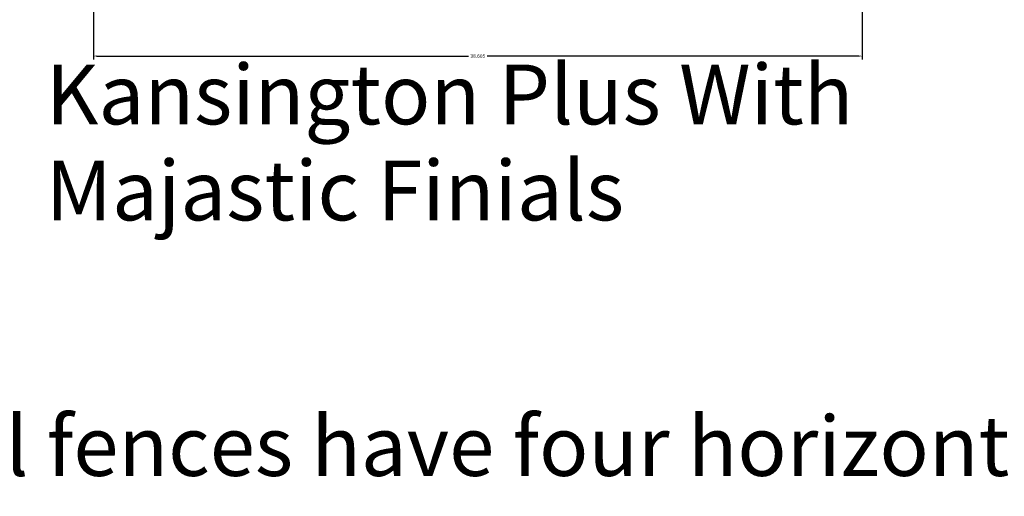
# Model space of a CAD drawing. Units: inches. Extents: x 756 to 915, y 488 to 695.
# Tile 4 of 25: x 813 to 863, y 488 to 512. Entities that reach past the tile are written whole.
import ezdxf

# ---------------------------------------------------------------- set-up
doc = ezdxf.new("R2010")
doc.units = ezdxf.units.IN
doc.header["$MEASUREMENT"] = 0
doc.layers.add('L-ANNO-TEXT', color=7, linetype='Continuous', lineweight=25)
doc.layers.add('M-DIMS', color=2, linetype='Continuous', lineweight=18)
doc.styles.get("Standard").update_dxf_attribs({"font": 'arial.ttf'})
doc.dimstyles.get("Standard").update_dxf_attribs({"dimtxt": 0.18, "dimasz": 0.18, "dimexe": 0.18, "dimexo": 0.0625, "dimgap": 0.09, "dimtad": 0, "dimtih": 1, "dimtoh": 1, "dimdec": 0, "dimzin": 0, "dimdsep": 46, "dimlunit": 3, "dimtxsty": 'Standard', "dimcen": 0.09, "dimadec": 0, "dimazin": 0, "dimtfac": 1, "dimtdec": 0, "dimtofl": 0, "dimtmove": 0, "dimatfit": 3, "dimfxl": 1, "dimtolj": 1, "dimtzin": 0, "dimarcsym": 0})

# ---------------------------------------------------------------- blocks, each defined once
blk = doc.blocks.new('*D78')
at = {"layer": 'Defpoints', "color": 0, "transparency": 16777216}
for p in [(817.069, 512.545), (855.674, 512.545), (855.674, 510.155)]:
    blk.add_point(p, dxfattribs=at)
at = {"layer": 'M-DIMS', "color": 0, "lineweight": -2, "transparency": 16777216}
for p, q in [((817.069, 512.482), (817.069, 509.975)), ((855.674, 512.482), (855.674, 509.975)), ((817.249, 510.155), (835.908, 510.155)), ((855.494, 510.155), (836.836, 510.155))]:
    blk.add_line(p, q, dxfattribs=at)
at = {"layer": 'M-DIMS', "color": 0, "transparency": 16777216}
for points in [[(817.249, 510.185), (817.249, 510.125), (817.069, 510.155)], [(855.494, 510.185), (855.494, 510.125), (855.674, 510.155)]]:
    blk.add_solid(points, dxfattribs=at)
at = {"layer": 'M-DIMS', "color": 0, "transparency": 16777216, "insert": (836.372, 510.155), "char_height": 0.18, "attachment_point": 5}
blk.add_mtext('\\A1;38.605', dxfattribs=at)

msp = doc.modelspace()

# ---------------------------------------------------------------- texts
at = {"layer": 'L-ANNO-TEXT'}
for s, p in [('Kansington Plus With', (814.6811, 506.7282)), ('Majastic Finials', (814.6811, 501.909)), ("6' high residential fences have four horizontal rails, not three as shown.", (779.8362, 489.0819))]:
    msp.add_text(s, height=3, dxfattribs=at).set_placement(p)

# ---------------------------------------------------------------- dimensions: what is measured, and where the dimension line sits
at = {"layer": 'M-DIMS'}
dim = msp.add_linear_dim(base=(855.6743, 510.1547), p1=(817.0694, 512.5447), p2=(855.6743, 512.5447), dimstyle='Standard', override={"dimdec": 3, "dimlfac": 1, "dimrnd": 0, "dimzin": 0, "dimdsep": 46, "dimlunit": 2}, dxfattribs=at)
dim.commit()
dim.dimension.update_dxf_attribs({"geometry": '*D78', "text_midpoint": (836.3719, 510.1547)})

doc.saveas('drawing.dxf')
